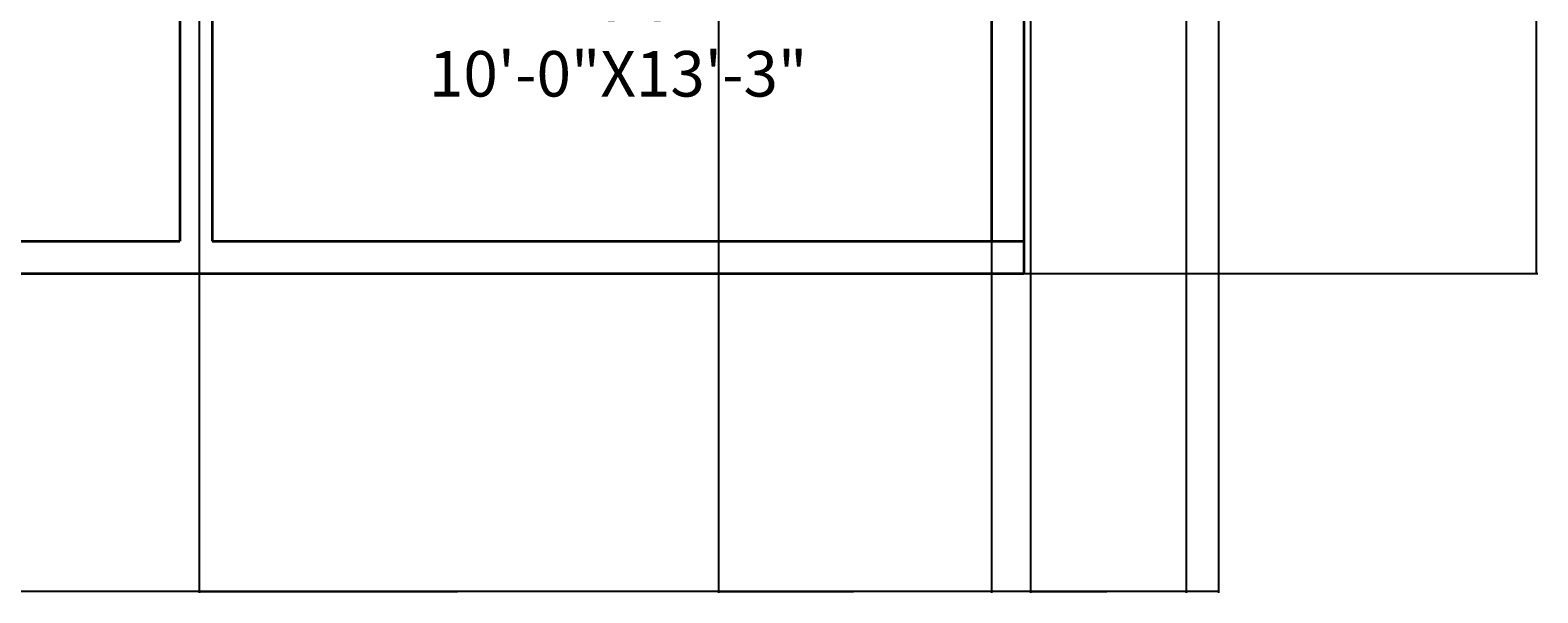
# Model space of a CAD drawing. Units: inches. Extents: x 3731 to 4318, y 1310 to 2388.
# Tile 15 of 57: x 4086 to 4318, y 1310 to 1397. Entities that reach past the tile are written whole.
import ezdxf

# ---------------------------------------------------------------- set-up
doc = ezdxf.new("R2010")
doc.units = ezdxf.units.IN
for name, color, linetype, lineweight in [('A-ANNO-DIMS', 2, 'Continuous', 18), ('A-AREA-IDEN', 7, 'Continuous', 18), ('A-WALL', 7, 'Continuous', 35)]:
    doc.layers.add(name, color=color, linetype=linetype, lineweight=lineweight)
doc.styles.get("Standard").update_dxf_attribs({"font": 'arial.ttf'})
doc.dimstyles.get("Standard").update_dxf_attribs({"dimtxt": 0.18, "dimasz": 0.18, "dimexe": 0.18, "dimexo": 0.0625, "dimgap": 0.09, "dimtad": 0, "dimtih": 1, "dimtoh": 1, "dimdec": 4, "dimzin": 0, "dimdsep": 46, "dimtxsty": 'Standard', "dimcen": 0.09, "dimadec": 0, "dimazin": 0, "dimtfac": 1, "dimtdec": 4, "dimtofl": 0, "dimtmove": 0, "dimatfit": 3, "dimfxl": 1, "dimtolj": 1, "dimtzin": 0, "dimarcsym": 0})

# ---------------------------------------------------------------- blocks, each defined once
blk = doc.blocks.new('*D32')
at = {"layer": 'A-ANNO-DIMS', "color": 0, "lineweight": -2, "transparency": 16777216}
for p, q in [((4269.21, 1592.32), (4269.21, 1310.25)), ((3835.21, 1359.32), (3835.21, 1310.25)), ((3835.39, 1310.43), (4051.92, 1310.43)), ((4269.03, 1310.43), (4052.5, 1310.43))]:
    blk.add_line(p, q, dxfattribs=at)
at = {"layer": 'A-ANNO-DIMS', "color": 0, "transparency": 16777216}
for points in [[(3835.39, 1310.46), (3835.39, 1310.4), (3835.21, 1310.43)], [(4269.03, 1310.46), (4269.03, 1310.4), (4269.21, 1310.43)]]:
    blk.add_solid(points, dxfattribs=at)
at = {"layer": 'Defpoints', "color": 0, "transparency": 16777216}
for p in [(4269.21, 1592.38), (3835.21, 1359.38), (4269.21, 1310.43)]:
    blk.add_point(p, dxfattribs=at)
at = {"layer": 'A-ANNO-DIMS', "color": 0, "transparency": 16777216, "insert": (4052.21, 1310.43), "char_height": 0.18, "attachment_point": 5}
blk.add_mtext('\\A1;434', dxfattribs=at)
blk = doc.blocks.new('*D42')
at = {"layer": 'A-ANNO-DIMS', "color": 0, "lineweight": -2, "transparency": 16777216}
for p, q in [((4269.27, 1592.38), (4318.34, 1592.38)), ((4318.16, 1592.2), (4318.16, 1476.06)), ((4318.16, 1359.56), (4318.16, 1475.7)), ((4239.27, 1359.38), (4318.34, 1359.38))]:
    blk.add_line(p, q, dxfattribs=at)
at = {"layer": 'A-ANNO-DIMS', "color": 0, "transparency": 16777216}
for points in [[(4318.13, 1592.2), (4318.19, 1592.2), (4318.16, 1592.38)], [(4318.13, 1359.56), (4318.19, 1359.56), (4318.16, 1359.38)]]:
    blk.add_solid(points, dxfattribs=at)
at = {"layer": 'Defpoints', "color": 0, "transparency": 16777216}
for p in [(4269.21, 1592.38), (4318.16, 1592.38), (4239.21, 1359.38)]:
    blk.add_point(p, dxfattribs=at)
at = {"layer": 'A-ANNO-DIMS', "color": 0, "transparency": 16777216, "insert": (4318.16, 1475.88), "char_height": 0.18, "attachment_point": 5}
blk.add_mtext('\\A1;233', dxfattribs=at)
blk = doc.blocks.new('*D43')
at = {"layer": 'A-ANNO-DIMS', "color": 0, "lineweight": -2, "transparency": 16777216}
for p, q in [((4240.21, 1597.39), (4240.21, 1310.25)), ((4264.21, 1597.32), (4264.21, 1310.25)), ((4240.39, 1310.43), (4251.99, 1310.43)), ((4264.03, 1310.43), (4252.43, 1310.43))]:
    blk.add_line(p, q, dxfattribs=at)
at = {"layer": 'A-ANNO-DIMS', "color": 0, "transparency": 16777216}
for points in [[(4240.39, 1310.46), (4240.39, 1310.4), (4240.21, 1310.43)], [(4264.03, 1310.46), (4264.03, 1310.4), (4264.21, 1310.43)]]:
    blk.add_solid(points, dxfattribs=at)
at = {"layer": 'Defpoints', "color": 0, "transparency": 16777216}
for p in [(4240.21, 1597.45), (4264.21, 1597.38), (4264.21, 1310.43)]:
    blk.add_point(p, dxfattribs=at)
at = {"layer": 'A-ANNO-DIMS', "color": 0, "transparency": 16777216, "insert": (4252.21, 1310.43), "char_height": 0.18, "attachment_point": 5}
blk.add_mtext('\\A1;24', dxfattribs=at)
blk = doc.blocks.new('*D46')
at = {"layer": 'A-ANNO-DIMS', "color": 0, "lineweight": -2, "transparency": 16777216}
for p, q in [((4112.21, 1854.32), (4112.21, 1310.25)), ((4192.21, 1854.32), (4192.21, 1310.25)), ((4112.39, 1310.43), (4151.99, 1310.43)), ((4192.03, 1310.43), (4152.43, 1310.43))]:
    blk.add_line(p, q, dxfattribs=at)
at = {"layer": 'A-ANNO-DIMS', "color": 0, "transparency": 16777216}
for points in [[(4112.39, 1310.46), (4112.39, 1310.4), (4112.21, 1310.43)], [(4192.03, 1310.46), (4192.03, 1310.4), (4192.21, 1310.43)]]:
    blk.add_solid(points, dxfattribs=at)
at = {"layer": 'Defpoints', "color": 0, "transparency": 16777216}
for p in [(4112.21, 1854.38), (4192.21, 1854.38), (4192.21, 1310.43)]:
    blk.add_point(p, dxfattribs=at)
at = {"layer": 'A-ANNO-DIMS', "color": 0, "transparency": 16777216, "insert": (4152.21, 1310.43), "char_height": 0.18, "attachment_point": 5}
blk.add_mtext('\\A1;80', dxfattribs=at)
blk = doc.blocks.new('*D47')
at = {"layer": 'A-ANNO-DIMS', "color": 0, "lineweight": -2, "transparency": 16777216}
for p, q in [((4192.21, 1854.32), (4192.21, 1310.25)), ((4234.21, 1854.32), (4234.21, 1310.25)), ((4192.39, 1310.43), (4212.99, 1310.43)), ((4234.03, 1310.43), (4213.43, 1310.43))]:
    blk.add_line(p, q, dxfattribs=at)
at = {"layer": 'A-ANNO-DIMS', "color": 0, "transparency": 16777216}
for points in [[(4192.39, 1310.46), (4192.39, 1310.4), (4192.21, 1310.43)], [(4234.03, 1310.46), (4234.03, 1310.4), (4234.21, 1310.43)]]:
    blk.add_solid(points, dxfattribs=at)
at = {"layer": 'Defpoints', "color": 0, "transparency": 16777216}
for p in [(4192.21, 1854.38), (4234.21, 1854.38), (4234.21, 1310.43)]:
    blk.add_point(p, dxfattribs=at)
at = {"layer": 'A-ANNO-DIMS', "color": 0, "transparency": 16777216, "insert": (4213.21, 1310.43), "char_height": 0.18, "attachment_point": 5}
blk.add_mtext('\\A1;42', dxfattribs=at)

msp = doc.modelspace()

# ---------------------------------------------------------------- linework, layer by layer
at = {"layer": 'A-WALL'}
for p, q in [((4239.21, 1592.38), (4239.21, 1359.38)), ((4234.21, 1527.38), (4234.21, 1364.38)), ((4109.21, 1491.38), (4109.21, 1364.38)), ((4114.21, 1491.38), (4114.21, 1364.38)), ((3947.21, 1364.38), (4109.21, 1364.38)), ((4114.21, 1364.38), (4239.21, 1364.38)), ((3942.21, 1359.38), (4239.21, 1359.38))]:
    msp.add_line(p, q, dxfattribs=at)

# ---------------------------------------------------------------- texts
at = {"layer": 'A-AREA-IDEN', "insert": (4147.6, 1405.28), "char_height": 7, "attachment_point": 1}
msp.add_mtext_dynamic_manual_height_columns('BEDROOM\\P10\'-0"X13\'-3"', width=47.0437, gutter_width=12.5, heights=[0], dxfattribs=at)

# ---------------------------------------------------------------- dimensions: what is measured, and where the dimension line sits
at = {"layer": 'A-ANNO-DIMS'}
for base, p1, p2, picture, middle in [((4192.21, 1310.43), (4112.21, 1854.38), (4192.21, 1854.38), '*D46', (4152.21, 1310.43)), ((4234.21, 1310.43), (4192.21, 1854.38), (4234.21, 1854.38), '*D47', (4213.21, 1310.43)), ((4264.21, 1310.43), (4240.21, 1597.45), (4264.21, 1597.38), '*D43', (4252.21, 1310.43)), ((4269.21, 1310.43), (3835.21, 1359.38), (4269.21, 1592.38), '*D32', (4052.21, 1310.43))]:
    dim = msp.add_linear_dim(base=base, p1=p1, p2=p2, dimstyle='Standard', override={"dimdec": 0, "dimlfac": 1, "dimrnd": 0, "dimzin": 0, "dimdsep": 46, "dimlunit": 2}, dxfattribs=at)
    dim.commit()
    dim.dimension.update_dxf_attribs({"geometry": picture, "text_midpoint": middle})
dim = msp.add_linear_dim(base=(4318.16, 1592.38), p1=(4239.21, 1359.38), p2=(4269.21, 1592.38), angle=90, dimstyle='Standard', override={"dimdec": 0, "dimlfac": 1, "dimrnd": 0, "dimzin": 0, "dimdsep": 46, "dimlunit": 2}, dxfattribs=at)
dim.commit()
dim.dimension.update_dxf_attribs({"geometry": '*D42', "text_midpoint": (4318.16, 1475.88)})

doc.saveas('drawing.dxf')
